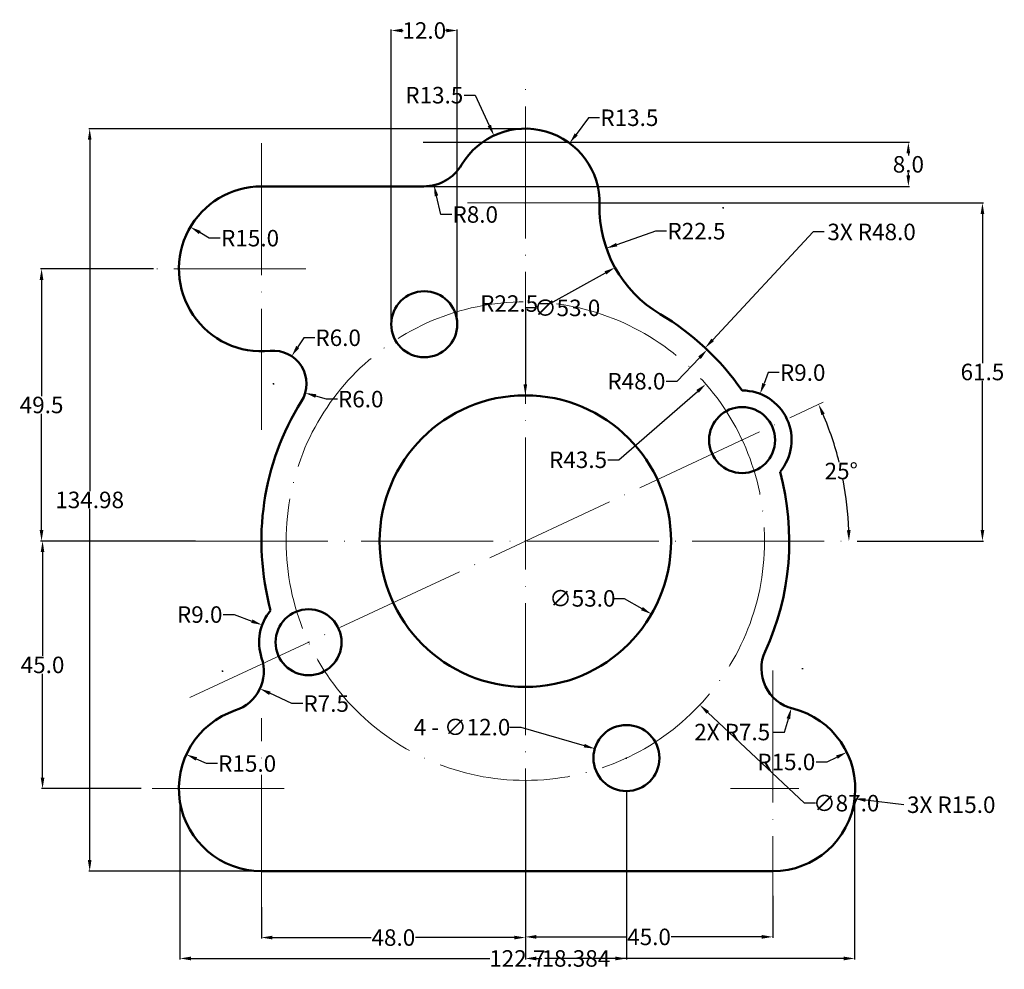
# Model space of a CAD drawing. Units: inches. Extents: x 215 to 394, y 87 to 260.
import ezdxf

# ---------------------------------------------------------------- set-up
doc = ezdxf.new("R2010")
doc.units = ezdxf.units.IN
doc.header["$MEASUREMENT"] = 0
doc.linetypes.add('ACAD_ISO04W100', pattern=[30, 24, -3, 0, -3])
for name, color, linetype, lineweight in [('M-CNTR', 4, 'ACAD_ISO04W100', 18), ('M-DIMS', 2, 'Continuous', 25), ('M-OUTL', 7, 'Continuous', 50)]:
    doc.layers.add(name, color=color, linetype=linetype, lineweight=lineweight)
doc.styles.get("Standard").update_dxf_attribs({"font": 'arial.ttf'})
doc.dimstyles.get("Standard").update_dxf_attribs({"dimtxt": 3, "dimasz": 2, "dimexe": 0.18, "dimexo": 0.0625, "dimgap": 0.09, "dimtad": 0, "dimtih": 1, "dimtoh": 1, "dimdec": 1, "dimzin": 0, "dimdsep": 46, "dimtxsty": 'Standard', "dimcen": 0.09, "dimadec": 0, "dimazin": 0, "dimtfac": 1, "dimtdec": 1, "dimtofl": 0, "dimtmove": 0, "dimatfit": 3, "dimfxl": 1, "dimtolj": 1, "dimtzin": 0, "dimarcsym": 0})

# ---------------------------------------------------------------- blocks, each defined once
blk = doc.blocks.new('*D1')
at = {"layer": 'Defpoints', "color": 0, "transparency": 16777216}
for p in [(365.38, 126.45), (351.92, 119.83)]:
    blk.add_point(p, dxfattribs=at)
at = {"layer": 'M-DIMS', "color": 0, "lineweight": -2, "transparency": 16777216}
for p, q in [((361.79, 124.68), (363.59, 125.57)), ((359.79, 124.68), (361.79, 124.68))]:
    blk.add_line(p, q, dxfattribs=at)
at = {"layer": 'M-DIMS', "color": 0, "transparency": 16777216}
blk.add_solid([(363.44, 125.86), (363.73, 125.27), (365.38, 126.45)], dxfattribs=at)
at = {"layer": 'M-DIMS', "color": 0, "transparency": 16777216, "insert": (354.38, 124.68), "char_height": 3, "attachment_point": 5}
blk.add_mtext('\\A1;R15.0', dxfattribs=at)
blk = doc.blocks.new('*D2')
at = {"layer": 'Defpoints', "color": 0, "transparency": 16777216}
for p in [(351.92, 100.38), (306.92, 99.47), (351.92, 92.88)]:
    blk.add_point(p, dxfattribs=at)
at = {"layer": 'M-DIMS', "color": 0, "lineweight": -2, "transparency": 16777216}
for p, q in [((351.92, 100.32), (351.92, 92.7)), ((306.92, 99.41), (306.92, 92.7)), ((308.92, 92.88), (325.38, 92.88)), ((349.92, 92.88), (333.46, 92.88))]:
    blk.add_line(p, q, dxfattribs=at)
at = {"layer": 'M-DIMS', "color": 0, "transparency": 16777216}
for points in [[(308.92, 93.22), (308.92, 92.55), (306.92, 92.88)], [(349.92, 93.22), (349.92, 92.55), (351.92, 92.88)]]:
    blk.add_solid(points, dxfattribs=at)
at = {"layer": 'M-DIMS', "color": 0, "transparency": 16777216, "insert": (329.42, 92.88), "char_height": 3, "attachment_point": 5}
blk.add_mtext('\\A1;45.0', dxfattribs=at)
blk = doc.blocks.new('*D3')
at = {"layer": 'Defpoints', "color": 0, "transparency": 16777216}
for p in [(306.92, 99.47), (258.92, 98.36), (258.92, 92.76)]:
    blk.add_point(p, dxfattribs=at)
at = {"layer": 'M-DIMS', "color": 0, "lineweight": -2, "transparency": 16777216}
for p, q in [((306.92, 99.41), (306.92, 92.58)), ((258.92, 98.29), (258.92, 92.58)), ((260.92, 92.76), (278.88, 92.76)), ((304.92, 92.76), (286.96, 92.76))]:
    blk.add_line(p, q, dxfattribs=at)
at = {"layer": 'M-DIMS', "color": 0, "transparency": 16777216}
for points in [[(260.92, 93.09), (260.92, 92.42), (258.92, 92.76)], [(304.92, 93.09), (304.92, 92.42), (306.92, 92.76)]]:
    blk.add_solid(points, dxfattribs=at)
at = {"layer": 'M-DIMS', "color": 0, "transparency": 16777216, "insert": (282.92, 92.76), "char_height": 3, "attachment_point": 5}
blk.add_mtext('\\A1;48.0', dxfattribs=at)
blk = doc.blocks.new('*D4')
at = {"layer": 'Defpoints', "color": 0, "transparency": 16777216}
for p in [(245.27, 126.05), (258.92, 119.83)]:
    blk.add_point(p, dxfattribs=at)
at = {"layer": 'M-DIMS', "color": 0, "lineweight": -2, "transparency": 16777216}
for p, q in [((248.91, 124.39), (247.09, 125.22)), ((250.91, 124.39), (248.91, 124.39))]:
    blk.add_line(p, q, dxfattribs=at)
at = {"layer": 'M-DIMS', "color": 0, "transparency": 16777216}
blk.add_solid([(247.23, 125.53), (246.95, 124.92), (245.27, 126.05)], dxfattribs=at)
at = {"layer": 'M-DIMS', "color": 0, "transparency": 16777216, "insert": (256.33, 124.39), "char_height": 3, "attachment_point": 5}
blk.add_mtext('\\A1;R15.0', dxfattribs=at)
blk = doc.blocks.new('*D5')
at = {"layer": 'Defpoints', "color": 0, "transparency": 16777216}
for p in [(251.86, 141.19), (258.65, 138.01)]:
    blk.add_point(p, dxfattribs=at)
at = {"layer": 'M-DIMS', "color": 0, "lineweight": -2, "transparency": 16777216}
for p, q in [((251.77, 141.19), (251.95, 141.19)), ((251.86, 141.1), (251.86, 141.28)), ((264.43, 135.3), (260.46, 137.16)), ((266.43, 135.3), (264.43, 135.3))]:
    blk.add_line(p, q, dxfattribs=at)
at = {"layer": 'M-DIMS', "color": 0, "transparency": 16777216}
blk.add_solid([(260.6, 137.46), (260.32, 136.86), (258.65, 138.01)], dxfattribs=at)
at = {"layer": 'M-DIMS', "color": 0, "transparency": 16777216, "insert": (270.7, 135.3), "char_height": 3, "attachment_point": 5}
blk.add_mtext('\\A1;R7.5', dxfattribs=at)
blk = doc.blocks.new('*D6')
at = {"layer": 'Defpoints', "color": 0, "transparency": 16777216}
for p in [(259.06, 149.58), (267.5, 146.44)]:
    blk.add_point(p, dxfattribs=at)
at = {"layer": 'M-DIMS', "color": 0, "lineweight": -2, "transparency": 16777216}
for p, q in [((251.95, 151.48), (253.95, 151.48)), ((253.95, 151.48), (257.19, 150.28)), ((267.41, 146.44), (267.59, 146.44)), ((267.5, 146.35), (267.5, 146.53))]:
    blk.add_line(p, q, dxfattribs=at)
at = {"layer": 'M-DIMS', "color": 0, "transparency": 16777216}
blk.add_solid([(257.3, 150.59), (257.07, 149.97), (259.06, 149.58)], dxfattribs=at)
at = {"layer": 'M-DIMS', "color": 0, "transparency": 16777216, "insert": (247.7, 151.48), "char_height": 3, "attachment_point": 5}
blk.add_mtext('\\A1;R9.0', dxfattribs=at)
blk = doc.blocks.new('*D7')
at = {"layer": 'Defpoints', "color": 0, "transparency": 16777216}
for p in [(246.98, 164.83), (219.12, 119.83), (237.09, 119.83)]:
    blk.add_point(p, dxfattribs=at)
at = {"layer": 'M-DIMS', "color": 0, "lineweight": -2, "transparency": 16777216}
for p, q in [((246.92, 164.83), (218.94, 164.83)), ((219.12, 162.83), (219.12, 143.95)), ((219.12, 121.83), (219.12, 140.71)), ((237.03, 119.83), (218.94, 119.83))]:
    blk.add_line(p, q, dxfattribs=at)
at = {"layer": 'M-DIMS', "color": 0, "transparency": 16777216}
for points in [[(218.78, 162.83), (219.45, 162.83), (219.12, 164.83)], [(218.78, 121.83), (219.45, 121.83), (219.12, 119.83)]]:
    blk.add_solid(points, dxfattribs=at)
at = {"layer": 'M-DIMS', "color": 0, "transparency": 16777216, "insert": (219.12, 142.33), "char_height": 3, "attachment_point": 5}
blk.add_mtext('\\A1;45.0', dxfattribs=at)
blk = doc.blocks.new('*D8')
at = {"layer": 'Defpoints', "color": 0, "transparency": 16777216}
for p in [(239.36, 214.33), (218.94, 164.83), (246.98, 164.83)]:
    blk.add_point(p, dxfattribs=at)
at = {"layer": 'M-DIMS', "color": 0, "lineweight": -2, "transparency": 16777216}
for p, q in [((239.3, 214.33), (218.76, 214.33)), ((218.94, 212.33), (218.94, 191.2)), ((218.94, 166.83), (218.94, 187.96)), ((246.92, 164.83), (218.76, 164.83))]:
    blk.add_line(p, q, dxfattribs=at)
at = {"layer": 'M-DIMS', "color": 0, "transparency": 16777216}
for points in [[(218.6, 212.33), (219.27, 212.33), (218.94, 214.33)], [(218.6, 166.83), (219.27, 166.83), (218.94, 164.83)]]:
    blk.add_solid(points, dxfattribs=at)
at = {"layer": 'M-DIMS', "color": 0, "transparency": 16777216, "insert": (218.94, 189.58), "char_height": 3, "attachment_point": 5}
blk.add_mtext('\\A1;49.5', dxfattribs=at)
blk = doc.blocks.new('*D9')
at = {"layer": 'Defpoints', "color": 0, "transparency": 16777216}
for p in [(320.42, 226.33), (367.18, 164.83), (390.05, 164.83)]:
    blk.add_point(p, dxfattribs=at)
at = {"layer": 'M-DIMS', "color": 0, "lineweight": -2, "transparency": 16777216}
for p, q in [((320.48, 226.33), (390.23, 226.33)), ((390.05, 224.33), (390.05, 197.2)), ((390.05, 166.83), (390.05, 193.96)), ((367.24, 164.83), (390.23, 164.83))]:
    blk.add_line(p, q, dxfattribs=at)
at = {"layer": 'M-DIMS', "color": 0, "transparency": 16777216}
for points in [[(389.72, 224.33), (390.38, 224.33), (390.05, 226.33)], [(389.72, 166.83), (390.38, 166.83), (390.05, 164.83)]]:
    blk.add_solid(points, dxfattribs=at)
at = {"layer": 'M-DIMS', "color": 0, "transparency": 16777216, "insert": (390.05, 195.58), "char_height": 3, "attachment_point": 5}
blk.add_mtext('\\A1;61.5', dxfattribs=at)
blk = doc.blocks.new('*D10')
at = {"layer": 'Defpoints', "color": 0, "transparency": 16777216}
for p in [(361.11, 190.1), (365.14, 173.36), (246.98, 164.83), (367.18, 164.83), (245.91, 136.38)]:
    blk.add_point(p, dxfattribs=at)
at = {"layer": 'M-DIMS', "color": 0, "lineweight": -2, "transparency": 16777216}
for start, end in [(14.1227, 23.0526), (1.9474, 10.8875)]:
    blk.add_arc((306.92, 164.83), 58.85, start, end, dxfattribs=at)
at = {"layer": 'M-DIMS', "color": 0, "transparency": 16777216}
for points in [[(360.76, 187.74), (361.37, 188.01), (360.25, 189.7)], [(366.07, 166.83), (365.4, 166.82), (365.77, 164.83)]]:
    blk.add_solid(points, dxfattribs=at)
at = {"layer": 'M-DIMS', "color": 0, "transparency": 16777216, "insert": (364.37, 177.57), "char_height": 3, "attachment_point": 5}
blk.add_mtext('\\A1;25°', dxfattribs=at)
blk = doc.blocks.new('*U11')
blk.add_circle((0, 0), 6)
blk = doc.blocks.new('*U12')
at = {"layer": 'M-OUTL', "color": 0, "linetype": 'ByBlock', "lineweight": -2, "transparency": 16777216}
for p, rotation in [((288.54, 204.25), 90.00000000000003), ((267.5, 146.44), 180), ((325.3, 125.4), 270.0000000000001)]:
    blk.add_blockref('*U11', p, dxfattribs=dict(at, rotation=rotation))
blk.add_blockref('*U11', (346.35, 183.21), dxfattribs=at)
blk = doc.blocks.new('*D13')
at = {"layer": 'Defpoints', "color": 0, "transparency": 16777216}
for p in [(264.43, 198.46), (261.13, 193.44)]:
    blk.add_point(p, dxfattribs=at)
at = {"layer": 'M-DIMS', "color": 0, "lineweight": -2, "transparency": 16777216}
for p, q in [((266.63, 201.8), (265.53, 200.13)), ((268.63, 201.8), (266.63, 201.8)), ((261.04, 193.44), (261.22, 193.44)), ((261.13, 193.35), (261.13, 193.53))]:
    blk.add_line(p, q, dxfattribs=at)
at = {"layer": 'M-DIMS', "color": 0, "transparency": 16777216}
blk.add_solid([(265.25, 200.31), (265.81, 199.94), (264.43, 198.46)], dxfattribs=at)
at = {"layer": 'M-DIMS', "color": 0, "transparency": 16777216, "insert": (272.88, 201.8), "char_height": 3, "attachment_point": 5}
blk.add_mtext('\\A1;R6.0', dxfattribs=at)
blk = doc.blocks.new('*D14')
at = {"layer": 'Defpoints', "color": 0, "transparency": 16777216}
for p in [(245.99, 221.94), (258.92, 214.33)]:
    blk.add_point(p, dxfattribs=at)
at = {"layer": 'M-DIMS', "color": 0, "lineweight": -2, "transparency": 16777216}
for p, q in [((249.44, 219.91), (247.72, 220.92)), ((251.44, 219.91), (249.44, 219.91))]:
    blk.add_line(p, q, dxfattribs=at)
at = {"layer": 'M-DIMS', "color": 0, "transparency": 16777216}
blk.add_solid([(247.89, 221.21), (247.55, 220.64), (245.99, 221.94)], dxfattribs=at)
at = {"layer": 'M-DIMS', "color": 0, "transparency": 16777216, "insert": (256.86, 219.91), "char_height": 3, "attachment_point": 5}
blk.add_mtext('\\A1;R15.0', dxfattribs=at)
blk = doc.blocks.new('*D15')
at = {"layer": 'Defpoints', "color": 0, "transparency": 16777216}
for p in [(288.45, 237.33), (290.3, 229.55)]:
    blk.add_point(p, dxfattribs=at)
at = {"layer": 'M-DIMS', "color": 0, "lineweight": -2, "transparency": 16777216}
for p, q in [((288.36, 237.33), (288.54, 237.33)), ((288.45, 237.24), (288.45, 237.42)), ((291.56, 224.21), (290.76, 227.6)), ((293.56, 224.21), (291.56, 224.21))]:
    blk.add_line(p, q, dxfattribs=at)
at = {"layer": 'M-DIMS', "color": 0, "transparency": 16777216}
blk.add_solid([(291.08, 227.68), (290.43, 227.52), (290.3, 229.55)], dxfattribs=at)
at = {"layer": 'M-DIMS', "color": 0, "transparency": 16777216, "insert": (297.81, 224.21), "char_height": 3, "attachment_point": 5}
blk.add_mtext('\\A1;R8.0', dxfattribs=at)
blk = doc.blocks.new('*D16')
at = {"layer": 'Defpoints', "color": 0, "transparency": 16777216}
for p in [(314.97, 237.17), (306.92, 226.33)]:
    blk.add_point(p, dxfattribs=at)
at = {"layer": 'M-DIMS', "color": 0, "lineweight": -2, "transparency": 16777216}
for p, q in [((318.41, 241.8), (316.16, 238.77)), ((320.41, 241.8), (318.41, 241.8)), ((306.83, 226.33), (307.01, 226.33)), ((306.92, 226.24), (306.92, 226.42))]:
    blk.add_line(p, q, dxfattribs=at)
at = {"layer": 'M-DIMS', "color": 0, "transparency": 16777216}
blk.add_solid([(315.89, 238.97), (316.43, 238.58), (314.97, 237.17)], dxfattribs=at)
at = {"layer": 'M-DIMS', "color": 0, "transparency": 16777216, "insert": (325.84, 241.8), "char_height": 3, "attachment_point": 5}
blk.add_mtext('\\A1;R13.5', dxfattribs=at)
blk = doc.blocks.new('*D17')
at = {"layer": 'Defpoints', "color": 0, "transparency": 16777216}
for p in [(342.91, 225.45), (321.66, 218.07)]:
    blk.add_point(p, dxfattribs=at)
at = {"layer": 'M-DIMS', "color": 0, "lineweight": -2, "transparency": 16777216}
for p, q in [((330.6, 221.18), (323.55, 218.72)), ((332.6, 221.18), (330.6, 221.18))]:
    blk.add_line(p, q, dxfattribs=at)
at = {"layer": 'M-DIMS', "color": 0, "transparency": 16777216}
blk.add_solid([(323.44, 219.04), (323.65, 218.41), (321.66, 218.07)], dxfattribs=at)
at = {"layer": 'M-DIMS', "color": 0, "transparency": 16777216, "insert": (338.04, 221.18), "char_height": 3, "attachment_point": 5}
blk.add_mtext('\\A1;R22.5', dxfattribs=at)
blk = doc.blocks.new('*D18')
at = {"layer": 'Defpoints', "color": 0, "transparency": 16777216}
for p in [(349.6, 191.6), (346.35, 183.21)]:
    blk.add_point(p, dxfattribs=at)
at = {"layer": 'M-DIMS', "color": 0, "lineweight": -2, "transparency": 16777216}
for p, q in [((351.11, 195.47), (350.33, 193.47)), ((353.11, 195.47), (351.11, 195.47)), ((346.26, 183.21), (346.44, 183.21)), ((346.35, 183.12), (346.35, 183.3))]:
    blk.add_line(p, q, dxfattribs=at)
at = {"layer": 'M-DIMS', "color": 0, "transparency": 16777216}
blk.add_solid([(350.02, 193.59), (350.64, 193.35), (349.6, 191.6)], dxfattribs=at)
at = {"layer": 'M-DIMS', "color": 0, "transparency": 16777216, "insert": (357.36, 195.47), "char_height": 3, "attachment_point": 5}
blk.add_mtext('\\A1;R9.0', dxfattribs=at)
blk = doc.blocks.new('*D19')
at = {"layer": 'Defpoints', "color": 0, "transparency": 16777216}
for p in [(339.98, 199.63), (306.92, 164.83)]:
    blk.add_point(p, dxfattribs=at)
at = {"layer": 'M-DIMS', "color": 0, "lineweight": -2, "transparency": 16777216}
for p, q in [((334.54, 193.9), (338.6, 198.18)), ((332.54, 193.9), (334.54, 193.9))]:
    blk.add_line(p, q, dxfattribs=at)
at = {"layer": 'M-DIMS', "color": 0, "transparency": 16777216}
blk.add_solid([(338.36, 198.41), (338.84, 197.95), (339.98, 199.63)], dxfattribs=at)
at = {"layer": 'M-DIMS', "color": 0, "transparency": 16777216, "insert": (327.12, 193.9), "char_height": 3, "attachment_point": 5}
blk.add_mtext('\\A1;R48.0', dxfattribs=at)
blk = doc.blocks.new('*D20')
at = {"layer": 'Defpoints', "color": 0, "transparency": 16777216}
for p in [(339.75, 193.37), (306.92, 164.83)]:
    blk.add_point(p, dxfattribs=at)
at = {"layer": 'M-DIMS', "color": 0, "lineweight": -2, "transparency": 16777216}
for p, q in [((323.94, 179.62), (338.24, 192.05)), ((321.94, 179.62), (323.94, 179.62))]:
    blk.add_line(p, q, dxfattribs=at)
at = {"layer": 'M-DIMS', "color": 0, "transparency": 16777216}
blk.add_solid([(338.02, 192.31), (338.46, 191.8), (339.75, 193.37)], dxfattribs=at)
at = {"layer": 'M-DIMS', "color": 0, "transparency": 16777216, "insert": (316.51, 179.62), "char_height": 3, "attachment_point": 5}
blk.add_mtext('\\A1;R43.5', dxfattribs=at)
blk = doc.blocks.new('*D21')
at = {"layer": 'Defpoints', "color": 0, "transparency": 16777216}
for p in [(319.54, 127.09), (331.06, 123.72)]:
    blk.add_point(p, dxfattribs=at)
at = {"layer": 'M-DIMS', "color": 0, "lineweight": -2, "transparency": 16777216}
for p, q in [((304.11, 131.01), (306.11, 131.01)), ((306.11, 131.01), (317.63, 127.65)), ((325.21, 125.4), (325.39, 125.4)), ((325.3, 125.31), (325.3, 125.49))]:
    blk.add_line(p, q, dxfattribs=at)
at = {"layer": 'M-DIMS', "color": 0, "transparency": 16777216}
blk.add_solid([(317.72, 127.97), (317.53, 127.33), (319.54, 127.09)], dxfattribs=at)
at = {"layer": 'M-DIMS', "color": 0, "transparency": 16777216, "insert": (295.41, 131.01), "char_height": 3, "attachment_point": 5}
blk.add_mtext('\\A1;4 - ∅12.0', dxfattribs=at)
blk = doc.blocks.new('*D22')
at = {"layer": 'Defpoints', "color": 0, "transparency": 16777216}
for p in [(283.98, 178.1), (329.86, 151.56)]:
    blk.add_point(p, dxfattribs=at)
at = {"layer": 'M-DIMS', "color": 0, "lineweight": -2, "transparency": 16777216}
for p, q in [((322.91, 154.42), (324.91, 154.42)), ((324.91, 154.42), (328.13, 152.56))]:
    blk.add_line(p, q, dxfattribs=at)
at = {"layer": 'M-DIMS', "color": 0, "transparency": 16777216}
blk.add_solid([(328.29, 152.85), (327.96, 152.27), (329.86, 151.56)], dxfattribs=at)
at = {"layer": 'M-DIMS', "color": 0, "transparency": 16777216, "insert": (317.29, 154.42), "char_height": 3, "attachment_point": 5}
blk.add_mtext('\\A1;∅53.0', dxfattribs=at)
blk = doc.blocks.new('*D23')
at = {"layer": 'Defpoints', "color": 0, "transparency": 16777216}
for p in [(244.11, 117.44), (366.81, 118), (366.81, 88.96)]:
    blk.add_point(p, dxfattribs=at)
at = {"layer": 'M-DIMS', "color": 0, "lineweight": -2, "transparency": 16777216}
for p, q in [((244.11, 117.38), (244.11, 88.78)), ((366.81, 117.94), (366.81, 88.78)), ((246.11, 88.96), (300.45, 88.96)), ((364.81, 88.96), (310.47, 88.96))]:
    blk.add_line(p, q, dxfattribs=at)
at = {"layer": 'M-DIMS', "color": 0, "transparency": 16777216}
for points in [[(246.11, 89.29), (246.11, 88.62), (244.11, 88.96)], [(364.81, 89.29), (364.81, 88.62), (366.81, 88.96)]]:
    blk.add_solid(points, dxfattribs=at)
at = {"layer": 'M-DIMS', "color": 0, "transparency": 16777216, "insert": (305.46, 88.96), "char_height": 3, "attachment_point": 5}
blk.add_mtext('\\A1;122.7', dxfattribs=at)
blk = doc.blocks.new('*D24')
at = {"layer": 'Defpoints', "color": 0, "transparency": 16777216}
for p in [(227.69, 239.81), (306.22, 239.81), (258.92, 104.83)]:
    blk.add_point(p, dxfattribs=at)
at = {"layer": 'M-DIMS', "color": 0, "lineweight": -2, "transparency": 16777216}
for p, q in [((306.16, 239.81), (227.51, 239.81)), ((227.69, 237.81), (227.69, 173.94)), ((227.69, 106.83), (227.69, 170.7)), ((258.86, 104.83), (227.51, 104.83))]:
    blk.add_line(p, q, dxfattribs=at)
at = {"layer": 'M-DIMS', "color": 0, "transparency": 16777216}
for points in [[(227.36, 237.81), (228.02, 237.81), (227.69, 239.81)], [(227.36, 106.83), (228.02, 106.83), (227.69, 104.83)]]:
    blk.add_solid(points, dxfattribs=at)
at = {"layer": 'M-DIMS', "color": 0, "transparency": 16777216, "insert": (227.69, 172.32), "char_height": 3, "attachment_point": 5}
blk.add_mtext('\\A1;134.98', dxfattribs=at)
blk = doc.blocks.new('*D25')
at = {"layer": 'Defpoints', "color": 0, "transparency": 16777216}
for p in [(306.92, 121.33), (325.3, 119.4), (325.3, 88.96)]:
    blk.add_point(p, dxfattribs=at)
at = {"layer": 'M-DIMS', "color": 0, "lineweight": -2, "transparency": 16777216}
for p, q in [((306.92, 121.27), (306.92, 88.78)), ((325.3, 119.34), (325.3, 88.78)), ((308.92, 88.96), (309.94, 88.96)), ((323.3, 88.96), (322.28, 88.96))]:
    blk.add_line(p, q, dxfattribs=at)
at = {"layer": 'M-DIMS', "color": 0, "transparency": 16777216}
for points in [[(308.92, 89.29), (308.92, 88.62), (306.92, 88.96)], [(323.3, 89.29), (323.3, 88.62), (325.3, 88.96)]]:
    blk.add_solid(points, dxfattribs=at)
at = {"layer": 'M-DIMS', "color": 0, "transparency": 16777216, "insert": (316.11, 88.96), "char_height": 3, "attachment_point": 5}
blk.add_mtext('\\A1;18.384', dxfattribs=at)
blk = doc.blocks.new('*D26')
at = {"layer": 'Defpoints', "color": 0, "transparency": 16777216}
for p in [(294.54, 257.66), (282.54, 204.25), (294.54, 204.25)]:
    blk.add_point(p, dxfattribs=at)
at = {"layer": 'M-DIMS', "color": 0, "lineweight": -2, "transparency": 16777216}
for p, q in [((282.54, 204.32), (282.54, 257.84)), ((284.54, 257.66), (284.7, 257.66)), ((292.54, 257.66), (292.38, 257.66)), ((294.54, 204.32), (294.54, 257.84))]:
    blk.add_line(p, q, dxfattribs=at)
at = {"layer": 'M-DIMS', "color": 0, "transparency": 16777216}
for points in [[(284.54, 257.99), (284.54, 257.32), (282.54, 257.66)], [(292.54, 257.99), (292.54, 257.32), (294.54, 257.66)]]:
    blk.add_solid(points, dxfattribs=at)
at = {"layer": 'M-DIMS', "color": 0, "transparency": 16777216, "insert": (288.54, 257.66), "char_height": 3, "attachment_point": 5}
blk.add_mtext('\\A1;12.0', dxfattribs=at)
blk = doc.blocks.new('*D27')
at = {"layer": 'Defpoints', "color": 0, "transparency": 16777216}
for p in [(288.45, 237.33), (288.45, 229.33), (376.58, 229.33)]:
    blk.add_point(p, dxfattribs=at)
at = {"layer": 'M-DIMS', "color": 0, "lineweight": -2, "transparency": 16777216}
for p, q in [((288.51, 237.33), (376.76, 237.33)), ((376.58, 235.33), (376.58, 234.95)), ((376.58, 231.33), (376.58, 231.71)), ((288.51, 229.33), (376.76, 229.33))]:
    blk.add_line(p, q, dxfattribs=at)
at = {"layer": 'M-DIMS', "color": 0, "transparency": 16777216}
for points in [[(376.24, 235.33), (376.91, 235.33), (376.58, 237.33)], [(376.24, 231.33), (376.91, 231.33), (376.58, 229.33)]]:
    blk.add_solid(points, dxfattribs=at)
at = {"layer": 'M-DIMS', "color": 0, "transparency": 16777216, "insert": (376.58, 233.33), "char_height": 3, "attachment_point": 5}
blk.add_mtext('\\A1;8.0', dxfattribs=at)
blk = doc.blocks.new('*D28')
at = {"layer": 'Defpoints', "color": 0, "transparency": 16777216}
for p in [(275.21, 194.6), (338.64, 135.06)]:
    blk.add_point(p, dxfattribs=at)
at = {"layer": 'M-DIMS', "color": 0, "lineweight": -2, "transparency": 16777216}
for p, q in [((306.83, 164.83), (307.01, 164.83)), ((306.92, 164.74), (306.92, 164.92)), ((357.67, 117.19), (340.09, 133.69)), ((359.67, 117.19), (357.67, 117.19))]:
    blk.add_line(p, q, dxfattribs=at)
at = {"layer": 'M-DIMS', "color": 0, "transparency": 16777216}
blk.add_solid([(340.32, 133.93), (339.87, 133.44), (338.64, 135.06)], dxfattribs=at)
at = {"layer": 'M-DIMS', "color": 0, "transparency": 16777216, "insert": (365.28, 117.19), "char_height": 3, "attachment_point": 5}
blk.add_mtext('\\A1;∅87.0', dxfattribs=at)
blk = doc.blocks.new('*D29')
at = {"layer": 'Defpoints', "color": 0, "transparency": 16777216}
for p in [(306.92, 191.33), (306.92, 138.33)]:
    blk.add_point(p, dxfattribs=at)
at = {"layer": 'M-DIMS', "color": 0, "lineweight": -2, "transparency": 16777216}
for p, q in [((308.92, 207.23), (306.92, 207.23)), ((306.92, 207.23), (306.92, 193.33)), ((306.83, 164.83), (307.01, 164.83)), ((306.92, 164.74), (306.92, 164.92))]:
    blk.add_line(p, q, dxfattribs=at)
at = {"layer": 'M-DIMS', "color": 0, "transparency": 16777216}
blk.add_solid([(306.59, 193.33), (307.25, 193.33), (306.92, 191.33)], dxfattribs=at)
at = {"layer": 'M-DIMS', "color": 0, "transparency": 16777216, "insert": (314.53, 207.23), "char_height": 3, "attachment_point": 5}
blk.add_mtext('\\A1;∅53.0', dxfattribs=at)
blk = doc.blocks.new('*D30')
at = {"layer": 'Defpoints', "color": 0, "transparency": 16777216}
for p in [(339.63, 199.96), (306.92, 164.83)]:
    blk.add_point(p, dxfattribs=at)
at = {"layer": 'M-DIMS', "color": 0, "lineweight": -2, "transparency": 16777216}
for p, q in [((359.25, 221.04), (340.99, 201.42)), ((361.25, 221.04), (359.25, 221.04)), ((306.83, 164.83), (307.01, 164.83)), ((306.92, 164.74), (306.92, 164.92))]:
    blk.add_line(p, q, dxfattribs=at)
at = {"layer": 'M-DIMS', "color": 0, "transparency": 16777216}
blk.add_solid([(340.75, 201.65), (341.24, 201.2), (339.63, 199.96)], dxfattribs=at)
at = {"layer": 'M-DIMS', "color": 0, "transparency": 16777216, "insert": (369.89, 221.04), "char_height": 3, "attachment_point": 5}
blk.add_mtext('\\A1;3X R48.0', dxfattribs=at)
blk = doc.blocks.new('*D31')
at = {"layer": 'Defpoints', "color": 0, "transparency": 16777216}
for p in [(342.91, 225.45), (323.22, 214.56)]:
    blk.add_point(p, dxfattribs=at)
at = {"layer": 'M-DIMS', "color": 0, "lineweight": -2, "transparency": 16777216}
for p, q in [((342.82, 225.45), (343, 225.45)), ((342.91, 225.36), (342.91, 225.54)), ((311.41, 208.02), (321.47, 213.59)), ((309.41, 208.02), (311.41, 208.02))]:
    blk.add_line(p, q, dxfattribs=at)
at = {"layer": 'M-DIMS', "color": 0, "transparency": 16777216}
blk.add_solid([(321.31, 213.88), (321.63, 213.3), (323.22, 214.56)], dxfattribs=at)
at = {"layer": 'M-DIMS', "color": 0, "transparency": 16777216, "insert": (303.98, 208.02), "char_height": 3, "attachment_point": 5}
blk.add_mtext('\\A1;R22.5', dxfattribs=at)
blk = doc.blocks.new('*D32')
at = {"layer": 'Defpoints', "color": 0, "transparency": 16777216}
for p in [(351.92, 119.83), (366.81, 118)]:
    blk.add_point(p, dxfattribs=at)
at = {"layer": 'M-DIMS', "color": 0, "lineweight": -2, "transparency": 16777216}
for p, q in [((351.83, 119.83), (352.01, 119.83)), ((351.92, 119.74), (351.92, 119.92)), ((375.74, 116.91), (368.79, 117.76))]:
    blk.add_line(p, q, dxfattribs=at)
at = {"layer": 'M-DIMS', "color": 0, "transparency": 16777216}
blk.add_solid([(368.83, 118.09), (368.75, 117.43), (366.81, 118)], dxfattribs=at)
at = {"layer": 'M-DIMS', "color": 0, "transparency": 16777216, "insert": (384.38, 116.91), "char_height": 3, "attachment_point": 5}
blk.add_mtext('\\A1;3X R15.0', dxfattribs=at)
blk = doc.blocks.new('*D33')
at = {"layer": 'Defpoints', "color": 0, "transparency": 16777216}
for p in [(301.22, 238.56), (306.92, 226.33)]:
    blk.add_point(p, dxfattribs=at)
at = {"layer": 'M-DIMS', "color": 0, "lineweight": -2, "transparency": 16777216}
for p, q in [((295.79, 245.9), (297.79, 245.9)), ((297.79, 245.9), (300.37, 240.38)), ((306.83, 226.33), (307.01, 226.33)), ((306.92, 226.24), (306.92, 226.42))]:
    blk.add_line(p, q, dxfattribs=at)
at = {"layer": 'M-DIMS', "color": 0, "transparency": 16777216}
blk.add_solid([(300.67, 240.52), (300.07, 240.24), (301.22, 238.56)], dxfattribs=at)
at = {"layer": 'M-DIMS', "color": 0, "transparency": 16777216, "insert": (290.36, 245.9), "char_height": 3, "attachment_point": 5}
blk.add_mtext('\\A1;R13.5', dxfattribs=at)
blk = doc.blocks.new('*D34')
at = {"layer": 'Defpoints', "color": 0, "transparency": 16777216}
for p in [(357.35, 141.66), (355.29, 134.45)]:
    blk.add_point(p, dxfattribs=at)
at = {"layer": 'M-DIMS', "color": 0, "lineweight": -2, "transparency": 16777216}
for p, q in [((357.26, 141.66), (357.44, 141.66)), ((357.35, 141.57), (357.35, 141.75)), ((354.06, 130.12), (354.75, 132.53)), ((352.06, 130.12), (354.06, 130.12))]:
    blk.add_line(p, q, dxfattribs=at)
at = {"layer": 'M-DIMS', "color": 0, "transparency": 16777216}
blk.add_solid([(354.42, 132.62), (355.07, 132.44), (355.29, 134.45)], dxfattribs=at)
at = {"layer": 'M-DIMS', "color": 0, "transparency": 16777216, "insert": (344.54, 130.12), "char_height": 3, "attachment_point": 5}
blk.add_mtext('\\A1;2X R7.5', dxfattribs=at)
blk = doc.blocks.new('*D35')
at = {"layer": 'Defpoints', "color": 0, "transparency": 16777216}
for p in [(261.13, 193.44), (266.89, 191.77)]:
    blk.add_point(p, dxfattribs=at)
at = {"layer": 'M-DIMS', "color": 0, "lineweight": -2, "transparency": 16777216}
for p, q in [((261.04, 193.44), (261.22, 193.44)), ((261.13, 193.35), (261.13, 193.53)), ((270.73, 190.65), (268.81, 191.21)), ((272.73, 190.65), (270.73, 190.65))]:
    blk.add_line(p, q, dxfattribs=at)
at = {"layer": 'M-DIMS', "color": 0, "transparency": 16777216}
blk.add_solid([(268.9, 191.53), (268.71, 190.89), (266.89, 191.77)], dxfattribs=at)
at = {"layer": 'M-DIMS', "color": 0, "transparency": 16777216, "insert": (276.98, 190.65), "char_height": 3, "attachment_point": 5}
blk.add_mtext('\\A1;R6.0', dxfattribs=at)

msp = doc.modelspace()

# ---------------------------------------------------------------- linework, layer by layer
at = {"layer": 'M-CNTR'}
for p, q in [((306.9207, 99.4708), (306.9207, 248.2558)), ((258.9207, 237.1669), (258.9207, 185.0383)), ((320.4207, 226.3288), (296.0693, 226.3288)), ((267.0174, 214.3288), (239.3597, 214.3288)), ((245.9113, 136.3797), (361.105, 190.0954)), ((246.9782, 164.8288), (367.1777, 164.8288)), ((351.9207, 141.3025), (351.9207, 100.3836)), ((258.9207, 98.3562), (258.9207, 132.6619)), ((263.0675, 119.8288), (237.0889, 119.8288)), ((356.6548, 119.8288), (344.2596, 119.8288))]:
    msp.add_line(p, q, dxfattribs=at)
msp.add_circle((306.9207, 164.8288), 43.5, dxfattribs=at)
at = {"layer": 'M-OUTL'}
for p, q in [((258.9207, 229.3288), (288.4477, 229.3288)), ((306.9207, 104.8288), (258.9207, 104.8288)), ((351.9207, 104.8288), (306.9207, 104.8288))]:
    msp.add_line(p, q, dxfattribs=at)
msp.add_circle((306.9207, 164.8288), 26.5, dxfattribs=at)
for centre, radius, start, end in [((306.9207, 226.3288), 13.5, 358.602403, 149.227675), ((288.4477, 237.3288), 8, 270, 329.227675), ((258.9207, 214.3288), 15, 90, 276.029163), ((342.91, 225.4508), 22.5, 178.602403, 239.303767), ((306.9207, 164.8288), 48, 34.784946, 59.303767), ((261.1264, 193.445), 6, 327.99935, 96.029163), ((346.3451, 183.2127), 9, 319.987074, 90.012926), ((306.9207, 164.8288), 48, 147.99935, 195.215054), ((306.9207, 164.8288), 48, 335.329072, 15.215054), ((267.4963, 146.4449), 9, 139.987074, 198.568533), ((251.8552, 141.1907), 7.5, 288.301677, 18.568533), ((357.3547, 141.6628), 7.5, 155.329072, 256.024347), ((351.9207, 119.8288), 15, 270, 76.024347), ((258.9207, 119.8288), 15, 108.301677, 270)]:
    msp.add_arc(centre, radius, start, end, dxfattribs=at)

# ---------------------------------------------------------------- block references
msp.add_blockref('*U12', (0, 0), dxfattribs=at)

# ---------------------------------------------------------------- dimensions: what is measured, and where the dimension line sits
at = {"layer": 'M-DIMS'}
for base, p1, p2, override, picture, middle in [((294.5368, 257.6558), (282.5368, 204.2532), (294.5368, 204.2532), {"dimdec": 1, "dimlfac": 1, "dimrnd": 0, "dimzin": 0, "dimdsep": 46, "dimlunit": 2}, '*D26', (288.5368, 257.6558)), ((325.3046, 88.9562), (306.9207, 121.3288), (325.3046, 119.4044), {"dimdec": 3, "dimlfac": 1, "dimrnd": 0, "dimzin": 0, "dimdsep": 46, "dimlunit": 2}, '*D25', (316.1126, 88.9562)), ((366.8093, 88.9562), (244.1116, 117.4433), (366.8093, 118.004), {"dimdec": 1, "dimlfac": 1, "dimrnd": 0, "dimzin": 0, "dimdsep": 46, "dimlunit": 2}, '*D23', (305.4604, 88.9562)), ((351.9207, 92.8841), (306.9207, 99.4708), (351.9207, 100.3836), {"dimclrd": 0, "dimclre": 0, "dimclrt": 0}, '*D2', (329.4207, 92.8841)), ((258.9207, 92.7557), (306.9207, 99.4708), (258.9207, 98.3562), {"dimclrd": 0, "dimclre": 0, "dimclrt": 0}, '*D3', (282.9207, 92.7557))]:
    dim = msp.add_linear_dim(base=base, p1=p1, p2=p2, dimstyle='Standard', override=override, dxfattribs=at)
    dim.commit()
    dim.dimension.update_dxf_attribs({"geometry": picture, "text_midpoint": middle})
for center, mpoint, override, picture, middle in [((306.9207, 226.3288), (301.2151, 238.5639), {"dimdec": 1, "dimlfac": 1, "dimrnd": 0, "dimzin": 0, "dimdsep": 46, "dimlunit": 2}, '*D33', (290.3586, 245.9049)), ((306.9207, 226.3288), (314.9681, 237.1681), {"dimclrd": 0, "dimclre": 0, "dimclrt": 0}, '*D16', (325.8386, 241.7979)), ((288.4477, 237.3288), (290.2952, 229.5451), {"dimclrd": 0, "dimclre": 0, "dimclrt": 0}, '*D15', (297.8126, 224.2106)), ((342.91, 225.4508), (323.222, 214.559), {"dimdec": 1, "dimlfac": 1, "dimrnd": 0, "dimzin": 0, "dimdsep": 46, "dimlunit": 2}, '*D31', (303.976, 208.0239)), ((342.91, 225.4508), (321.6557, 218.0679), {"dimclrd": 0, "dimclre": 0, "dimclrt": 0}, '*D17', (338.0351, 221.1755)), ((258.9207, 214.3288), (245.9945, 221.939), {"dimclrd": 0, "dimclre": 0, "dimclrt": 0}, '*D14', (256.8582, 219.9096)), ((306.9207, 164.8288), (339.9804, 199.6291), {"dimclrd": 0, "dimclre": 0, "dimclrt": 0}, '*D19', (327.1209, 193.8998)), ((346.3451, 183.2127), (349.6039, 191.602), {"dimclrd": 0, "dimclre": 0, "dimclrt": 0}, '*D18', (357.3593, 195.4738)), ((306.9207, 164.8288), (339.7514, 193.3664), {"dimclrd": 0, "dimclre": 0, "dimclrt": 0}, '*D20', (316.5086, 179.6241)), ((267.4963, 146.4449), (259.0609, 149.5824), {"dimclrd": 0, "dimclre": 0, "dimclrt": 0}, '*D6', (247.7003, 151.4827)), ((251.8552, 141.1907), (258.6464, 138.0078), {"dimclrd": 0, "dimclre": 0, "dimclrt": 0}, '*D5', (270.7012, 135.2955)), ((258.9207, 119.8288), (245.2733, 126.0537), {"dimclrd": 0, "dimclre": 0, "dimclrt": 0}, '*D4', (256.3294, 124.3938)), ((351.9207, 119.8288), (365.3813, 126.4478), {"dimclrd": 0, "dimclre": 0, "dimclrt": 0}, '*D1', (354.3751, 124.6827))]:
    dim = msp.add_radius_dim(center=center, mpoint=mpoint, dimstyle='Standard', override=override, dxfattribs=at)
    dim.commit()
    dim.dimension.update_dxf_attribs({"geometry": picture, "text_midpoint": middle, "dimtype": 164})
for base, p1, p2, override, picture, middle in [((227.6889, 239.8117), (258.9207, 104.8288), (306.2179, 239.8117), {"dimdec": 2, "dimlfac": 1, "dimrnd": 0, "dimzin": 0, "dimdsep": 46, "dimlunit": 2}, '*D24', (227.6889, 172.3203)), ((376.5777, 229.3288), (288.4477, 237.3288), (288.4477, 229.3288), {"dimdec": 1, "dimlfac": 1, "dimrnd": 0, "dimzin": 0, "dimdsep": 46, "dimlunit": 2}, '*D27', (376.5777, 233.3288)), ((390.0501, 164.8288), (320.4207, 226.3288), (367.1777, 164.8288), {"dimclrd": 0, "dimclre": 0, "dimclrt": 0}, '*D9', (390.0501, 195.5788)), ((218.9376, 164.8288), (239.3597, 214.3288), (246.9782, 164.8288), {"dimclrd": 0, "dimclre": 0, "dimclrt": 0}, '*D8', (218.9376, 189.5788)), ((219.1176, 119.8288), (246.9782, 164.8288), (237.0889, 119.8288), {"dimclrd": 0, "dimclre": 0, "dimclrt": 0}, '*D7', (219.1176, 142.3288))]:
    dim = msp.add_linear_dim(base=base, p1=p1, p2=p2, angle=90, dimstyle='Standard', override=override, dxfattribs=at)
    dim.commit()
    dim.dimension.update_dxf_attribs({"geometry": picture, "text_midpoint": middle})
for center, mpoint, text, picture, middle in [((306.9207, 164.8288), (339.6293, 199.9593), '3X <>', '*D30', (369.8932, 221.0376)), ((357.3547, 141.6628), (355.2946, 134.4513), '2X <>', '*D34', (344.5423, 130.1243)), ((351.9207, 119.8288), (366.8093, 118.004), '3X <>', '*D32', (375.7424, 116.909))]:
    dim = msp.add_radius_dim(center=center, mpoint=mpoint, text=text, dimstyle='Standard', override={"dimdec": 1, "dimlfac": 1, "dimrnd": 0, "dimzin": 0, "dimdsep": 46, "dimlunit": 2}, dxfattribs=at)
    dim.commit()
    dim.dimension.update_dxf_attribs({"geometry": picture, "text_midpoint": middle, "dimtype": 164})
for p1, p2, override, picture, middle in [((306.9204, 138.3288), (306.921, 191.3288), {"dimdec": 1, "dimlfac": 1, "dimrnd": 0, "dimzin": 0, "dimdsep": 46, "dimlunit": 2}, '*D29', (314.5344, 207.2288)), ((275.2053, 194.6011), (338.636, 135.0566), {"dimdec": 1, "dimlfac": 1, "dimrnd": 0, "dimzin": 0, "dimdsep": 46, "dimlunit": 2}, '*D28', (365.2784, 117.1932)), ((283.9824, 178.0986), (329.859, 151.5591), {"dimclrd": 0, "dimclre": 0, "dimclrt": 0}, '*D22', (317.2941, 154.4236))]:
    dim = msp.add_diameter_dim_2p(p1=p1, p2=p2, dimstyle='Standard', override=override, dxfattribs=at)
    dim.commit()
    dim.dimension.update_dxf_attribs({"geometry": picture, "text_midpoint": middle, "dimtype": 163})
for mpoint, override, picture, middle in [((264.4279, 198.455), {"dimclrd": 0, "dimclre": 0, "dimclrt": 0}, '*D13', (272.8802, 201.795)), ((266.8876, 191.7691), {"dimdec": 1, "dimlfac": 1, "dimrnd": 0, "dimzin": 0, "dimdsep": 46, "dimlunit": 2}, '*D35', (276.9797, 190.6518))]:
    dim = msp.add_radius_dim(center=(261.1264, 193.445), mpoint=mpoint, dimstyle='Standard', override=override, dxfattribs=at)
    dim.commit()
    dim.dimension.update_dxf_attribs({"geometry": picture, "text_midpoint": middle})
dim = msp.add_angular_dim_2l(base=(365.1448, 173.3574), line1=((246.9782, 164.8288), (367.1777, 164.8288)), line2=((245.9113, 136.3797), (361.105, 190.0954)), dimstyle='Standard', override={"dimclrd": 0, "dimclre": 0, "dimclrt": 0}, dxfattribs=at)
dim.commit()
dim.dimension.update_dxf_attribs({"geometry": '*D10', "text_midpoint": (364.3712, 177.5653)})
dim = msp.add_diameter_dim_2p(p1=(331.0642, 123.7231), p2=(319.545, 127.0857), text='4 - <>', dimstyle='Standard', override={"dimclrd": 0, "dimclre": 0, "dimclrt": 0}, dxfattribs=at)
dim.commit()
dim.dimension.update_dxf_attribs({"geometry": '*D21', "text_midpoint": (295.414, 131.0066), "dimtype": 163})

doc.saveas('drawing.dxf')
